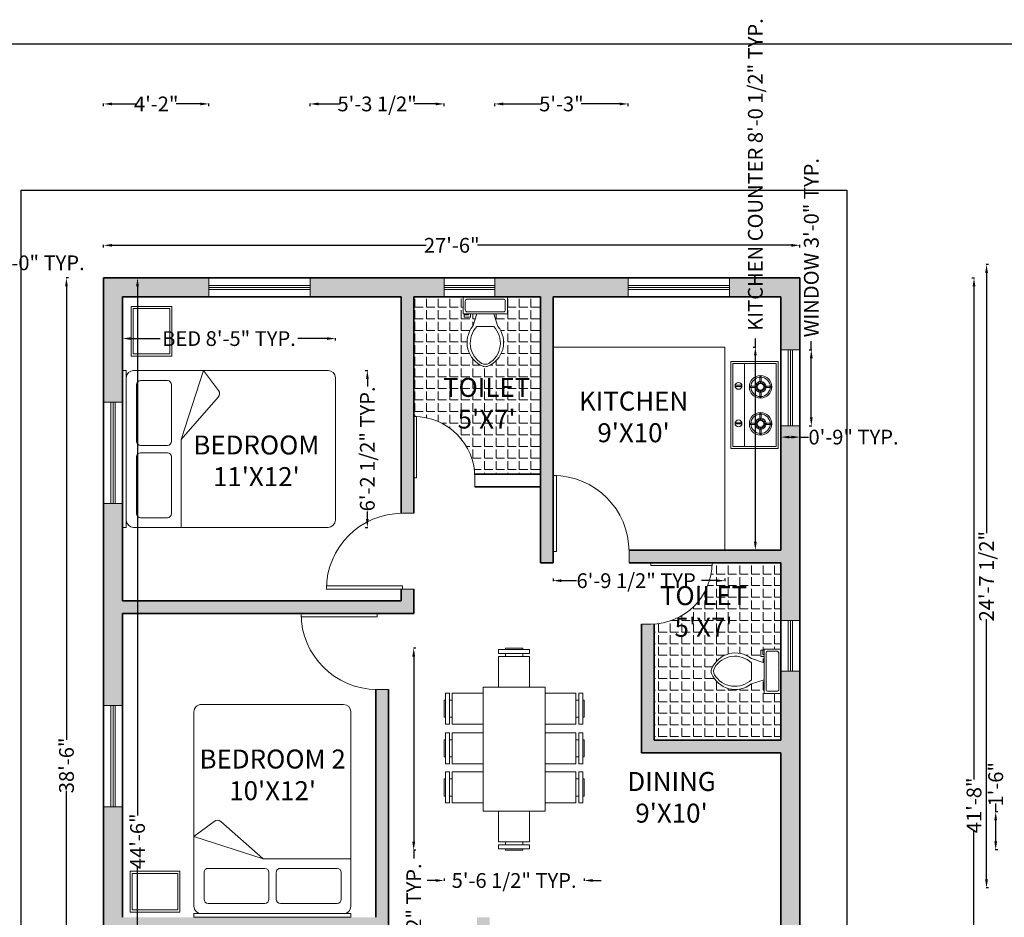
# Model space of a CAD drawing. Units: inches. Extents: x -80 to 1461, y -1239 to 153.
# Tile 5 of 6: x 358 to 824, y -273 to 153. Entities that reach past the tile are written whole.
import ezdxf

# ---------------------------------------------------------------- set-up
doc = ezdxf.new("R2010")
doc.units = ezdxf.units.IN
doc.header["$MEASUREMENT"] = 0
for name, color, linetype, lineweight in [('A-ANNO-DIMS', 2, 'Continuous', 18), ('A-ANNO-TTLB', 7, 'Continuous', 25), ('A-AREA-IDEN', 7, 'Continuous', 18), ('A-EQPM', 8, 'Continuous', 18), ('A-FLOR-FIXT', 9, 'Continuous', 18), ('A-FLOR-PATT', 143, 'Continuous', 13), ('A-FURN', 8, 'Continuous', 18), ('A-GLAZ', 4, 'Continuous', 18), ('A-WALL', 7, 'Continuous', 35), ('A-WALL-PATT', 8, 'Continuous', 13), ('DOOR', 32, 'Continuous', 18)]:
    doc.layers.add(name, color=color, linetype=linetype, lineweight=lineweight)
doc.styles.get("Standard").update_dxf_attribs({"font": 'arial.ttf'})
doc.dimstyles.get("Standard").update_dxf_attribs({"dimtxt": 7, "dimasz": 4, "dimexe": 0.18, "dimexo": 0.0625, "dimgap": 0.09, "dimtad": 0, "dimdec": 0, "dimzin": 0, "dimdsep": 46, "dimlunit": 3, "dimtxsty": 'Standard', "dimcen": 0.09, "dimadec": 0, "dimazin": 0, "dimtfac": 1, "dimtdec": 0, "dimtofl": 0, "dimtmove": 0, "dimatfit": 3, "dimfxl": 1, "dimfxlon": 1, "dimtolj": 1, "dimtzin": 0, "dimarcsym": 0})

# ---------------------------------------------------------------- blocks, each defined once
blk = doc.blocks.new('*U2')
for p, q in [((0, 0), (0, -6)), ((40, 0), (40, -6))]:
    blk.add_line(p, q)
blk.add_lwpolyline([(0, 0), (0, 40), (1.75, 40), (1.75, 0)], close=True)
blk.add_arc((0, 0), 40, 0, 90)
blk = doc.blocks.new('A$C164346CA')
for p, q in [((0, 2.035), (0, 2)), ((1.5, 2.035), (0, 2.035)), ((1.5, 2), (0, 2)), ((1.5, 2), (1.5, 2.035)), ((0, 1.93), (0, 0.07)), ((0.6731, 1.9024), (0.1319, 1.9024)), ((1.364, 1.9024), (0.8228, 1.9024)), ((1.5, 0.07), (1.5, 1.93)), ((0.0919, 1.8624), (0.0919, 1.6069)), ((0.7131, 1.6069), (0.7131, 1.8624)), ((0.7828, 1.8624), (0.7828, 1.6069)), ((1.404, 1.6069), (1.404, 1.8624)), ((0.1319, 1.5669), (0.6731, 1.5669)), ((0.8228, 1.5669), (1.364, 1.5669)), ((0.8395, 1.4761), (0, 1.4761)), ((0.8395, 1.4761), (1.2448, 1.12)), ((1.5, 1.2611), (0.8395, 1.4761)), ((1.3077, 1.1175), (1.5, 1.2611)), ((0.07, 0), (1.43, 0))]:
    blk.add_line(p, q)
for centre, radius, start, end in [((0.07, 1.93), 0.07, 90, 180), ((1.43, 1.93), 0.07, 0, 90), ((0.1319, 1.8624), 0.04, 90, 180), ((0.6731, 1.8624), 0.04, 0, 90), ((0.8228, 1.8624), 0.04, 90, 180), ((1.364, 1.8624), 0.04, 0, 90), ((0.1319, 1.6069), 0.04, 180, 270), ((0.6731, 1.6069), 0.04, 270, 0), ((0.8228, 1.6069), 0.04, 180, 270), ((1.364, 1.6069), 0.04, 270, 0), ((1.2778, 1.1575), 0.05, 228.69584, 306.75789), ((0.07, 0.07), 0.07, 180, 270), ((1.43, 0.07), 0.07, 270, 0)]:
    blk.add_arc(centre, radius, start, end)
blk = doc.blocks.new('*U5')
for p, q in [((241, -152), (241, -51)), ((-254, -216), (-203, -216)), ((-254, -241), (-254, -216)), ((-203, -216), (-203, -203)), ((-178, -203), (-178, -241)), ((-102, -203), (-152, -356)), ((102, -203), (152, -356)), ((-178, -241), (-254, -241)), ((102, -356), (-102, -356))]:
    blk.add_line(p, q)
blk.add_lwpolyline([(267, -203), (267, 0), (-267, 0), (-267, -203)], close=True)
for points in [[(-241, -51), (-241, -152)], [(216, -25), (-216, -25)], [(-216, -178), (216, -178)]]:
    blk.add_lwpolyline(points)
for centre, radius, start, end in [((-219, -48), 22.5, 81.8699, 188.1301), ((219, -48), 22.5, 351.8699, 98.1301), ((-219, -156), 22.5, 171.8699, 278.1301), ((219, -156), 22.5, 261.8699, 8.1301), ((89, -548), 309, 141.4691, 247.9714), ((107, -554), 288, 136.3677, 238.9468), ((-89, -548), 309, 292.0284, 38.5307), ((-107, -554), 288, 301.053, 43.6321), ((0, -708), 102, 245.7318, 294.2682), ((0, -737), 102, 254.8605, 285.1395)]:
    blk.add_arc(centre, radius, start, end)
blk = doc.blocks.new('A$C06E242FC')
for p, q in [((0, 455.6), (0.5, 456.1)), ((0, 455.6), (0, 0.5)), ((838.9, 456.1), (0.5, 456.1)), ((20, 435.6), (20.5, 436.1)), ((20, 435.6), (20, 20.5)), ((818.9, 436.1), (20.5, 436.1)), ((237.3, 411.5), (237.3, 356.2)), ((248.9, 411.5), (237.3, 411.5)), ((248.9, 356.2), (248.9, 411.5)), ((599.3, 411.5), (610.9, 411.5)), ((599.3, 411.5), (599.3, 356.2)), ((610.9, 356.2), (610.9, 411.5)), ((819.4, 435.6), (818.9, 436.1)), ((819.4, 20.5), (819.4, 435.6)), ((838.9, 456.1), (839.4, 455.6)), ((839.4, 0.5), (839.4, 455.6)), ((20, 324.4), (819.4, 324.4)), ((237.3, 356.2), (248.9, 356.2)), ((599.3, 356.2), (610.9, 356.2)), ((232.7, 272.7), (232.7, 214)), ((244.9, 272.7), (232.7, 272.7)), ((232.7, 214), (244.9, 214)), ((244.9, 214), (244.9, 272.7)), ((588.1, 272.7), (588.1, 214)), ((600.3, 272.7), (588.1, 272.7)), ((588.1, 214), (600.3, 214)), ((600.3, 214), (600.3, 272.7)), ((136.3, 176), (136.3, 163.8)), ((194.9, 176), (136.3, 176)), ((136.3, 163.8), (194.9, 163.8)), ((194.9, 163.8), (194.9, 176)), ((245.2, 126.1), (233, 126.1)), ((233, 126.1), (233, 67.4)), ((245.2, 67.4), (245.2, 126.1)), ((282.9, 176.3), (282.9, 164.1)), ((341.6, 176.3), (282.9, 176.3)), ((282.9, 164.1), (341.6, 164.1)), ((341.6, 164.1), (341.6, 176.3)), ((550.3, 176), (491.7, 176)), ((491.7, 176), (491.7, 163.8)), ((491.7, 163.8), (550.3, 163.8)), ((550.3, 163.8), (550.3, 176)), ((600.6, 126.1), (588.3, 126.1)), ((588.3, 126.1), (588.3, 67.4)), ((600.6, 67.4), (600.6, 126.1)), ((638.3, 176.3), (638.3, 164.1)), ((697, 176.3), (638.3, 176.3)), ((638.3, 164.1), (697, 164.1)), ((697, 164.1), (697, 176.3)), ((0, 0.5), (0.5, 0)), ((20, 20.5), (20.5, 20)), ((20.5, 20), (818.9, 20)), ((233, 67.4), (245.2, 67.4)), ((588.3, 67.4), (600.6, 67.4)), ((818.9, 20), (819.4, 20.5)), ((838.9, 0), (839.4, 0.5)), ((0.5, 0), (838.9, 0))]:
    blk.add_line(p, q)
for centre, radius in [((242, 382.9), 33.3), ((604.1, 382.9), 33.3), ((238.9, 170.1), 108.3), ((238.9, 170.1), 93.3), ((238.9, 170.1), 52.6), ((205.3, 189.5), 4.84), ((238.9, 170.1), 32.6), ((219.5, 203.7), 4.84), ((238.9, 208.9), 4.84), ((258.4, 203.7), 4.84), ((272.6, 189.5), 4.84), ((594.3, 170.1), 108.3), ((594.3, 170.1), 93.3), ((594.3, 170.1), 52.6), ((560.7, 189.5), 4.84), ((594.3, 170.1), 32.6), ((574.9, 203.7), 4.84), ((594.3, 208.9), 4.84), ((613.7, 203.7), 4.84), ((628, 189.5), 4.84), ((200.1, 170.1), 4.84), ((205.3, 150.6), 4.84), ((219.5, 136.4), 4.84), ((238.9, 131.2), 4.84), ((258.4, 136.4), 4.84), ((272.6, 150.6), 4.84), ((277.8, 170.1), 4.84), ((555.5, 170.1), 4.84), ((560.7, 150.6), 4.84), ((574.9, 136.4), 4.84), ((594.3, 131.2), 4.84), ((613.7, 136.4), 4.84), ((628, 150.6), 4.84), ((633.2, 170.1), 4.84)]:
    blk.add_circle(centre, radius)
blk = doc.blocks.new('A$C4C0603CD')
for p, q in [((1.106, 2.02), (0.656, 2.02)), ((0.656, 2.02), (0.656, 1.96)), ((1.006, 2.04), (0.756, 2.04)), ((0.756, 2.04), (0.756, 2.02)), ((1.006, 2.02), (1.006, 2.04)), ((1.106, 1.96), (1.106, 2.02)), ((1.232, 2.02), (1.232, 1.96)), ((1.684, 2.02), (1.232, 2.02)), ((1.584, 2.04), (1.334, 2.04)), ((1.334, 2.04), (1.334, 2.02)), ((1.584, 2.02), (1.584, 2.04)), ((1.684, 1.96), (1.684, 2.02)), ((1.802, 2.02), (1.802, 1.96)), ((2.252, 2.02), (1.802, 2.02)), ((2.152, 2.04), (1.902, 2.04)), ((1.902, 2.04), (1.902, 2.02)), ((2.152, 2.02), (2.152, 2.04)), ((2.252, 1.96), (2.252, 2.02)), ((1.106, 1.96), (0.656, 1.96)), ((0.656, 1.92), (0.656, 1.47)), ((1.106, 1.92), (0.656, 1.92)), ((0.756, 1.96), (0.756, 1.92)), ((1.006, 1.92), (1.006, 1.96)), ((1.106, 1.47), (1.106, 1.92)), ((1.684, 1.96), (1.232, 1.96)), ((1.232, 1.92), (1.232, 1.47)), ((1.684, 1.92), (1.232, 1.92)), ((1.334, 1.96), (1.334, 1.92)), ((1.584, 1.92), (1.584, 1.96)), ((1.684, 1.47), (1.684, 1.92)), ((2.252, 1.96), (1.802, 1.96)), ((1.802, 1.92), (1.802, 1.47)), ((2.252, 1.92), (1.802, 1.92)), ((1.902, 1.96), (1.902, 1.92)), ((2.152, 1.92), (2.152, 1.96)), ((2.252, 1.47), (2.252, 1.92)), ((0.57, 1.47), (0.57, 0.57)), ((2.37, 1.47), (0.57, 1.47)), ((0.656, 1.47), (1.106, 1.47)), ((1.107, 1.47), (1.684, 1.47)), ((1.802, 1.47), (2.252, 1.47)), ((2.37, 1.47), (2.37, 0.57)), ((0.02, 1.245), (0.02, 0.795)), ((0.08, 1.245), (0.02, 1.245)), ((0.08, 1.245), (0.08, 0.795)), ((0.12, 1.245), (0.12, 0.795)), ((0.57, 1.245), (0.12, 1.245)), ((0.57, 0.795), (0.57, 1.245)), ((2.37, 1.245), (2.37, 0.795)), ((2.82, 1.245), (2.37, 1.245)), ((2.82, 0.795), (2.82, 1.245)), ((2.86, 0.795), (2.86, 1.245)), ((2.92, 1.245), (2.86, 1.245)), ((2.92, 0.795), (2.92, 1.245)), ((0, 1.145), (0, 0.895)), ((0.02, 1.145), (0, 1.145)), ((0.12, 1.145), (0.08, 1.145)), ((2.86, 1.145), (2.82, 1.145)), ((2.94, 1.145), (2.92, 1.145)), ((2.94, 0.895), (2.94, 1.145)), ((0, 0.895), (0.02, 0.895)), ((0.08, 0.895), (0.12, 0.895)), ((2.82, 0.895), (2.86, 0.895)), ((2.92, 0.895), (2.94, 0.895)), ((0.02, 0.795), (0.08, 0.795)), ((0.12, 0.795), (0.57, 0.795)), ((2.37, 0.795), (2.82, 0.795)), ((2.86, 0.795), (2.92, 0.795)), ((0.57, 0.57), (2.37, 0.57)), ((1.106, 0.57), (0.656, 0.57)), ((0.656, 0.57), (0.656, 0.12)), ((1.106, 0.12), (1.106, 0.57)), ((1.684, 0.57), (1.232, 0.57)), ((1.232, 0.57), (1.232, 0.12)), ((1.684, 0.12), (1.684, 0.57)), ((2.252, 0.57), (1.802, 0.57)), ((1.802, 0.57), (1.802, 0.12)), ((2.252, 0.12), (2.252, 0.57)), ((0.656, 0.12), (1.106, 0.12)), ((0.656, 0.08), (1.106, 0.08)), ((0.656, 0.08), (0.656, 0.02)), ((0.656, 0.02), (1.106, 0.02)), ((0.756, 0.12), (0.756, 0.08)), ((0.756, 0.02), (0.756, 0)), ((0.756, 0), (1.006, 0)), ((1.006, 0.08), (1.006, 0.12)), ((1.006, 0), (1.006, 0.02)), ((1.106, 0.02), (1.106, 0.08)), ((1.232, 0.12), (1.684, 0.12)), ((1.232, 0.08), (1.684, 0.08)), ((1.232, 0.08), (1.232, 0.02)), ((1.232, 0.02), (1.684, 0.02)), ((1.334, 0.12), (1.334, 0.08)), ((1.334, 0.02), (1.334, 0)), ((1.334, 0), (1.584, 0)), ((1.584, 0.08), (1.584, 0.12)), ((1.584, 0), (1.584, 0.02)), ((1.684, 0.02), (1.684, 0.08)), ((1.802, 0.12), (2.252, 0.12)), ((1.802, 0.08), (2.252, 0.08)), ((1.802, 0.08), (1.802, 0.02)), ((1.802, 0.02), (2.252, 0.02)), ((1.902, 0.12), (1.902, 0.08)), ((1.902, 0.02), (1.902, 0)), ((1.902, 0), (2.152, 0)), ((2.152, 0.08), (2.152, 0.12)), ((2.152, 0), (2.152, 0.02)), ((2.252, 0.02), (2.252, 0.08))]:
    blk.add_line(p, q)
blk = doc.blocks.new('*D13')
at = {"layer": 'A-ANNO-DIMS', "color": 0, "lineweight": -2, "transparency": 16777216}
for p, q in [((397.42, 44.81), (397.42, 45.99)), ((401.42, 45.81), (550.24, 45.81)), ((723.42, 45.81), (574.59, 45.81)), ((727.42, 44.81), (727.42, 45.99))]:
    blk.add_line(p, q, dxfattribs=at)
at = {"layer": 'A-ANNO-DIMS', "color": 0, "transparency": 16777216}
for points in [[(401.42, 46.47), (401.42, 45.14), (397.42, 45.81)], [(723.42, 46.47), (723.42, 45.14), (727.42, 45.81)]]:
    blk.add_solid(points, dxfattribs=at)
at = {"layer": 'Defpoints', "color": 0, "transparency": 16777216}
for p in [(727.42, 45.81), (397.42, 30.32), (727.42, 30.32)]:
    blk.add_point(p, dxfattribs=at)
at = {"layer": 'A-ANNO-DIMS', "color": 0, "transparency": 16777216, "insert": (562.42, 45.81), "char_height": 7, "attachment_point": 5}
blk.add_mtext('\\A1;27\'-6"', dxfattribs=at)
blk = doc.blocks.new('*D14')
at = {"layer": 'A-ANNO-DIMS', "color": 0, "lineweight": -2, "transparency": 16777216}
for p, q in [((380.82, 30.32), (379.64, 30.32)), ((379.82, 26.32), (379.82, -188.57)), ((379.82, -427.68), (379.82, -212.8)), ((380.82, -431.68), (379.64, -431.68))]:
    blk.add_line(p, q, dxfattribs=at)
at = {"layer": 'A-ANNO-DIMS', "color": 0, "transparency": 16777216}
for points in [[(379.15, 26.32), (380.48, 26.32), (379.82, 30.32)], [(379.15, -427.68), (380.48, -427.68), (379.82, -431.68)]]:
    blk.add_solid(points, dxfattribs=at)
at = {"layer": 'Defpoints', "color": 0, "transparency": 16777216}
for p in [(397.42, 30.32), (379.82, -431.68), (397.42, -431.68)]:
    blk.add_point(p, dxfattribs=at)
at = {"layer": 'A-ANNO-DIMS', "color": 0, "transparency": 16777216, "insert": (379.82, -200.68), "char_height": 7, "attachment_point": 5, "rotation": 90}
blk.add_mtext('\\A1;38\'-6"', dxfattribs=at)
blk = doc.blocks.new('*D21')
at = {"layer": 'A-ANNO-DIMS', "color": 0, "lineweight": -2, "transparency": 16777216}
for p, q in [((820.21, -222.68), (820.21, -218.68)), ((821.21, -222.68), (820.03, -222.68)), ((820.21, -236.68), (820.21, -226.68)), ((821.21, -240.68), (820.03, -240.68))]:
    blk.add_line(p, q, dxfattribs=at)
at = {"layer": 'A-ANNO-DIMS', "color": 0, "transparency": 16777216}
for points in [[(819.55, -226.68), (820.88, -226.68), (820.21, -222.68)], [(819.55, -236.68), (820.88, -236.68), (820.21, -240.68)]]:
    blk.add_solid(points, dxfattribs=at)
at = {"layer": 'Defpoints', "color": 0, "transparency": 16777216}
for p in [(820.21, -222.68), (841.26, -222.68), (838.26, -240.68)]:
    blk.add_point(p, dxfattribs=at)
at = {"layer": 'A-ANNO-DIMS', "color": 0, "transparency": 16777216, "insert": (820.21, -209.62), "char_height": 7, "attachment_point": 5, "rotation": 90}
blk.add_mtext('\\A1;1\'-6"', dxfattribs=at)
blk = doc.blocks.new('WIN-48IN')
for p, q in [((0, 9), (0, 0)), ((48, 9), (0, 9)), ((0, 5.5), (48, 5.5)), ((48, 0), (48, 9)), ((0, 4.5), (48, 4.5)), ((0, 3.5), (48, 3.5)), ((0, 0), (36, 0)), ((36, 0), (48, 0))]:
    blk.add_line(p, q)
blk = doc.blocks.new('WIN-24IN')
for p, q in [((0, 9), (0, 0)), ((0, 9), (24, 9)), ((0, 5.5), (24, 5.5)), ((24, 9), (24, 0)), ((0, 4.5), (24, 4.5)), ((0, 3.5), (24, 3.5)), ((0, 0), (24, 0))]:
    blk.add_line(p, q)
blk = doc.blocks.new('WIN-36IN')
for p, q in [((0, 36), (9, 36)), ((0, 36), (0, 0)), ((3.5, 0), (3.5, 36)), ((4.5, 0), (4.5, 36)), ((5.5, 0), (5.5, 36)), ((9, 0), (9, 36)), ((0, 0), (9, 0))]:
    blk.add_line(p, q)
blk = doc.blocks.new('NIGHTSTAND')
for points in [[(0, 19.36), (23.56, 19.36), (23.56, 0), (0, 0)], [(1, 18.36), (22.56, 18.36), (22.56, 1), (1, 1)]]:
    blk.add_lwpolyline(points, close=True)
blk = doc.blocks.new('COUNTER-L-PLAN')
for p, q in [((0, 96.29), (81.45, 96.29)), ((81.45, 96.29), (81.45, 0))]:
    blk.add_line(p, q)
blk = doc.blocks.new('*D36')
at = {"layer": 'A-ANNO-DIMS', "color": 0, "lineweight": -2, "transparency": 16777216}
for p, q in [((249.57, 36.52), (249.57, 37.7)), ((253.57, 37.52), (293.57, 37.52)), ((297.57, 36.52), (297.57, 37.7)), ((297.57, 37.52), (301.57, 37.52))]:
    blk.add_line(p, q, dxfattribs=at)
at = {"layer": 'A-ANNO-DIMS', "color": 0, "transparency": 16777216}
for points in [[(253.57, 38.18), (253.57, 36.85), (249.57, 37.52)], [(293.57, 38.18), (293.57, 36.85), (297.57, 37.52)]]:
    blk.add_solid(points, dxfattribs=at)
at = {"layer": 'Defpoints', "color": 0, "transparency": 16777216}
for p in [(297.57, 37.52), (249.57, 30.32), (297.57, 30.32)]:
    blk.add_point(p, dxfattribs=at)
at = {"layer": 'A-ANNO-DIMS', "color": 0, "transparency": 16777216, "insert": (345.95, 37.52), "char_height": 7, "attachment_point": 5}
blk.add_mtext('\\A1;WINDOW 4\'-0" TYP.', dxfattribs=at)
blk = doc.blocks.new('*D40')
at = {"layer": 'A-ANNO-DIMS', "color": 0, "lineweight": -2, "transparency": 16777216}
for p, q in [((732.82, -3.69), (732.82, 0.31)), ((731.82, -3.69), (733, -3.69)), ((732.82, -35.69), (732.82, -7.69)), ((731.82, -39.69), (733, -39.69))]:
    blk.add_line(p, q, dxfattribs=at)
at = {"layer": 'A-ANNO-DIMS', "color": 0, "transparency": 16777216}
for points in [[(732.15, -7.69), (733.48, -7.69), (732.82, -3.69)], [(732.15, -35.69), (733.48, -35.69), (732.82, -39.69)]]:
    blk.add_solid(points, dxfattribs=at)
at = {"layer": 'Defpoints', "color": 0, "transparency": 16777216}
for p in [(727.42, -3.69), (732.82, -3.69), (727.42, -39.69)]:
    blk.add_point(p, dxfattribs=at)
at = {"layer": 'A-ANNO-DIMS', "color": 0, "transparency": 16777216, "insert": (732.82, 44.69), "char_height": 7, "attachment_point": 5, "rotation": 90}
blk.add_mtext('\\A1;WINDOW 3\'-0" TYP.', dxfattribs=at)
blk = doc.blocks.new('*D41')
at = {"layer": 'A-ANNO-DIMS', "color": 0, "lineweight": -2, "transparency": 16777216}
for p, q in [((718.42, -44.09), (718.42, -45.27)), ((722.42, -45.09), (723.42, -45.09)), ((727.42, -44.09), (727.42, -45.27)), ((727.42, -45.09), (731.42, -45.09))]:
    blk.add_line(p, q, dxfattribs=at)
at = {"layer": 'A-ANNO-DIMS', "color": 0, "transparency": 16777216}
for points in [[(722.42, -44.42), (722.42, -45.76), (718.42, -45.09)], [(723.42, -44.42), (723.42, -45.76), (727.42, -45.09)]]:
    blk.add_solid(points, dxfattribs=at)
at = {"layer": 'Defpoints', "color": 0, "transparency": 16777216}
for p in [(718.42, -39.69), (727.42, -39.69), (727.42, -45.09)]:
    blk.add_point(p, dxfattribs=at)
at = {"layer": 'A-ANNO-DIMS', "color": 0, "transparency": 16777216, "insert": (752.84, -45.09), "char_height": 7, "attachment_point": 5}
blk.add_mtext('\\A1;0\'-9" TYP.', dxfattribs=at)
blk = doc.blocks.new('*D46')
at = {"layer": 'A-ANNO-DIMS', "color": 0, "lineweight": -2, "transparency": 16777216}
for p, q in [((406.42, 0.62), (406.42, 1.8)), ((410.42, 1.62), (424.17, 1.62)), ((503.29, 1.62), (489.53, 1.62)), ((507.29, 0.62), (507.29, 1.8))]:
    blk.add_line(p, q, dxfattribs=at)
at = {"layer": 'A-ANNO-DIMS', "color": 0, "transparency": 16777216}
for points in [[(410.42, 2.29), (410.42, 0.96), (406.42, 1.62)], [(503.29, 2.29), (503.29, 0.96), (507.29, 1.62)]]:
    blk.add_solid(points, dxfattribs=at)
at = {"layer": 'Defpoints', "color": 0, "transparency": 16777216}
for p in [(406.42, 1.62), (406.42, -13.51), (507.29, -13.51)]:
    blk.add_point(p, dxfattribs=at)
at = {"layer": 'A-ANNO-DIMS', "color": 0, "transparency": 16777216, "insert": (456.85, 1.62), "char_height": 7, "attachment_point": 5}
blk.add_mtext('\\A1;BED 8\'-5" TYP.', dxfattribs=at)
blk = doc.blocks.new('*D47')
at = {"layer": 'A-ANNO-DIMS', "color": 0, "lineweight": -2, "transparency": 16777216}
for p, q in [((521.42, -13.51), (522.6, -13.51)), ((522.42, -17.51), (522.42, -21.09)), ((522.42, -83.86), (522.42, -80.28)), ((521.42, -87.86), (522.6, -87.86))]:
    blk.add_line(p, q, dxfattribs=at)
at = {"layer": 'A-ANNO-DIMS', "color": 0, "transparency": 16777216}
for points in [[(521.75, -17.51), (523.08, -17.51), (522.42, -13.51)], [(521.75, -83.86), (523.08, -83.86), (522.42, -87.86)]]:
    blk.add_solid(points, dxfattribs=at)
at = {"layer": 'Defpoints', "color": 0, "transparency": 16777216}
for p in [(507.29, -13.51), (522.42, -13.51), (507.29, -87.86)]:
    blk.add_point(p, dxfattribs=at)
at = {"layer": 'A-ANNO-DIMS', "color": 0, "transparency": 16777216, "insert": (522.42, -50.68), "char_height": 7, "attachment_point": 5, "rotation": 90}
blk.add_mtext('\\A1;6\'-2 1/2" TYP.', dxfattribs=at)
blk = doc.blocks.new('*D52')
at = {"layer": 'A-ANNO-DIMS', "color": 0, "lineweight": -2, "transparency": 16777216}
for p, q in [((545.39, -145.12), (544.21, -145.12)), ((544.39, -149.12), (544.39, -236.86)), ((545.39, -240.86), (544.21, -240.86)), ((544.39, -240.86), (544.39, -244.86))]:
    blk.add_line(p, q, dxfattribs=at)
at = {"layer": 'A-ANNO-DIMS', "color": 0, "transparency": 16777216}
for points in [[(543.72, -149.12), (545.06, -149.12), (544.39, -145.12)], [(543.72, -236.86), (545.06, -236.86), (544.39, -240.86)]]:
    blk.add_solid(points, dxfattribs=at)
at = {"layer": 'Defpoints', "color": 0, "transparency": 16777216}
for p in [(558.75, -145.12), (544.39, -240.86), (558.75, -240.86)]:
    blk.add_point(p, dxfattribs=at)
at = {"layer": 'A-ANNO-DIMS', "color": 0, "transparency": 16777216, "insert": (544.39, -306.33), "char_height": 7, "attachment_point": 5, "rotation": 90}
blk.add_mtext('\\A1;DINING SET 7\'-11 1/2" TYP.', dxfattribs=at)
blk = doc.blocks.new('*D53')
at = {"layer": 'A-ANNO-DIMS', "color": 0, "lineweight": -2, "transparency": 16777216}
for p, q in [((554.75, -255.23), (550.75, -255.23)), ((558.75, -254.23), (558.75, -255.41)), ((625.19, -254.23), (625.19, -255.41)), ((629.19, -255.23), (633.19, -255.23))]:
    blk.add_line(p, q, dxfattribs=at)
at = {"layer": 'A-ANNO-DIMS', "color": 0, "transparency": 16777216}
for points in [[(554.75, -254.56), (554.75, -255.89), (558.75, -255.23)], [(629.19, -254.56), (629.19, -255.89), (625.19, -255.23)]]:
    blk.add_solid(points, dxfattribs=at)
at = {"layer": 'Defpoints', "color": 0, "transparency": 16777216}
for p in [(558.75, -240.86), (625.19, -240.86), (625.19, -255.23)]:
    blk.add_point(p, dxfattribs=at)
at = {"layer": 'A-ANNO-DIMS', "color": 0, "transparency": 16777216, "insert": (591.97, -255.23), "char_height": 7, "attachment_point": 5}
blk.add_mtext('\\A1;5\'-6 1/2" TYP.', dxfattribs=at)
blk = doc.blocks.new('*D60')
at = {"layer": 'A-ANNO-DIMS', "color": 0, "lineweight": -2, "transparency": 16777216}
for p, q in [((706.3, -2.4), (706.3, 1.6)), ((705.3, -2.4), (706.48, -2.4)), ((706.3, -94.68), (706.3, -6.4)), ((705.3, -98.68), (706.48, -98.68))]:
    blk.add_line(p, q, dxfattribs=at)
at = {"layer": 'A-ANNO-DIMS', "color": 0, "transparency": 16777216}
for points in [[(705.64, -6.4), (706.97, -6.4), (706.3, -2.4)], [(705.64, -94.68), (706.97, -94.68), (706.3, -98.68)]]:
    blk.add_solid(points, dxfattribs=at)
at = {"layer": 'Defpoints', "color": 0, "transparency": 16777216}
for p in [(691.86, -2.4), (706.3, -2.4), (691.86, -98.68)]:
    blk.add_point(p, dxfattribs=at)
at = {"layer": 'A-ANNO-DIMS', "color": 0, "transparency": 16777216, "insert": (706.3, 79.38), "char_height": 7, "attachment_point": 5, "rotation": 90}
blk.add_mtext('\\A1;KITCHEN COUNTER 8\'-0 1/2" TYP.', dxfattribs=at)
blk = doc.blocks.new('*D61')
at = {"layer": 'A-ANNO-DIMS', "color": 0, "lineweight": -2, "transparency": 16777216}
for p, q in [((610.42, -112.13), (610.42, -113.31)), ((614.42, -113.13), (621.54, -113.13)), ((687.86, -113.13), (680.74, -113.13)), ((691.86, -112.13), (691.86, -113.31))]:
    blk.add_line(p, q, dxfattribs=at)
at = {"layer": 'A-ANNO-DIMS', "color": 0, "transparency": 16777216}
for points in [[(614.42, -112.46), (614.42, -113.79), (610.42, -113.13)], [(687.86, -112.46), (687.86, -113.79), (691.86, -113.13)]]:
    blk.add_solid(points, dxfattribs=at)
at = {"layer": 'Defpoints', "color": 0, "transparency": 16777216}
for p in [(610.42, -98.68), (691.86, -98.68), (691.86, -113.13)]:
    blk.add_point(p, dxfattribs=at)
at = {"layer": 'A-ANNO-DIMS', "color": 0, "transparency": 16777216, "insert": (651.14, -113.13), "char_height": 7, "attachment_point": 5}
blk.add_mtext('\\A1;6\'-9 1/2" TYP.', dxfattribs=at)
blk = doc.blocks.new('*D63')
at = {"layer": 'A-ANNO-DIMS', "color": 0, "lineweight": -2, "transparency": 16777216}
for p, q in [((816.86, 36.65), (815.68, 36.65)), ((815.86, 32.65), (815.86, -90.69)), ((815.86, -254.68), (815.86, -131.34)), ((816.86, -258.68), (815.68, -258.68))]:
    blk.add_line(p, q, dxfattribs=at)
at = {"layer": 'A-ANNO-DIMS', "color": 0, "transparency": 16777216}
for points in [[(815.2, 32.65), (816.53, 32.65), (815.86, 36.65)], [(815.2, -254.68), (816.53, -254.68), (815.86, -258.68)]]:
    blk.add_solid(points, dxfattribs=at)
at = {"layer": 'Defpoints', "color": 0, "transparency": 16777216}
for p in [(815.86, 36.65), (847.26, 36.65), (835.26, -258.68)]:
    blk.add_point(p, dxfattribs=at)
at = {"layer": 'A-ANNO-DIMS', "color": 0, "transparency": 16777216, "insert": (815.86, -111.02), "char_height": 7, "attachment_point": 5, "rotation": 90}
blk.add_mtext('\\A1;24\'-7 1/2"', dxfattribs=at)
blk = doc.blocks.new('*D72')
at = {"layer": 'A-ANNO-DIMS', "color": 0, "lineweight": -2, "transparency": 16777216}
for p, q in [((412.49, 30.32), (413.67, 30.32)), ((413.49, 26.32), (413.49, -224.38)), ((413.49, -499.58), (413.49, -248.89)), ((412.49, -503.58), (413.67, -503.58))]:
    blk.add_line(p, q, dxfattribs=at)
at = {"layer": 'A-ANNO-DIMS', "color": 0, "transparency": 16777216}
for points in [[(412.82, 26.32), (414.16, 26.32), (413.49, 30.32)], [(412.82, -499.58), (414.16, -499.58), (413.49, -503.58)]]:
    blk.add_solid(points, dxfattribs=at)
at = {"layer": 'Defpoints', "color": 0, "transparency": 16777216}
for p in [(330.99, 30.32), (183.99, -503.58), (413.49, -503.58)]:
    blk.add_point(p, dxfattribs=at)
at = {"layer": 'A-ANNO-DIMS', "color": 0, "transparency": 16777216, "insert": (413.49, -236.63), "char_height": 7, "attachment_point": 5, "rotation": 90}
blk.add_mtext('\\A1;44\'-6"', dxfattribs=at)
blk = doc.blocks.new('*D73')
at = {"layer": 'A-ANNO-DIMS', "color": 0, "lineweight": -2, "transparency": 16777216}
for p, q in [((808.92, 30.32), (810.1, 30.32)), ((809.92, 26.32), (809.92, -207.38)), ((809.92, -465.58), (809.92, -231.89)), ((808.92, -469.58), (810.1, -469.58))]:
    blk.add_line(p, q, dxfattribs=at)
at = {"layer": 'A-ANNO-DIMS', "color": 0, "transparency": 16777216}
for points in [[(809.25, 26.32), (810.58, 26.32), (809.92, 30.32)], [(809.25, -465.58), (810.58, -465.58), (809.92, -469.58)]]:
    blk.add_solid(points, dxfattribs=at)
at = {"layer": 'Defpoints', "color": 0, "transparency": 16777216}
for p in [(727.42, 30.32), (809.92, 30.32), (580.42, -469.58)]:
    blk.add_point(p, dxfattribs=at)
at = {"layer": 'A-ANNO-DIMS', "color": 0, "transparency": 16777216, "insert": (809.92, -219.63), "char_height": 7, "attachment_point": 5, "rotation": 90}
blk.add_mtext('\\A1;41\'-8"', dxfattribs=at)
blk = doc.blocks.new('*D77')
at = {"layer": 'A-ANNO-DIMS', "color": 0, "lineweight": -2, "transparency": 16777216}
for p, q in [((610.42, -500.08), (610.42, -501.26)), ((614.42, -501.08), (619.02, -501.08)), ((642.42, -501.08), (637.81, -501.08)), ((646.42, -500.08), (646.42, -501.26))]:
    blk.add_line(p, q, dxfattribs=at)
at = {"layer": 'A-ANNO-DIMS', "color": 0, "transparency": 16777216}
for points in [[(614.42, -500.42), (614.42, -501.75), (610.42, -501.08)], [(642.42, -500.42), (642.42, -501.75), (646.42, -501.08)]]:
    blk.add_solid(points, dxfattribs=at)
at = {"layer": 'Defpoints', "color": 0, "transparency": 16777216}
for p in [(610.42, -104.68), (646.42, -104.68), (646.42, -501.08)]:
    blk.add_point(p, dxfattribs=at)
at = {"layer": 'A-ANNO-DIMS', "color": 0, "transparency": 16777216, "insert": (628.42, -501.08), "char_height": 7, "attachment_point": 5}
blk.add_mtext('\\A1;3\'-0"', dxfattribs=at)
blk = doc.blocks.new('*D78')
at = {"layer": 'A-ANNO-DIMS', "color": 0, "lineweight": -2, "transparency": 16777216}
for p, q in [((397.42, 111.82), (397.42, 113)), ((401.42, 112.82), (412.81, 112.82)), ((443.28, 112.82), (431.88, 112.82)), ((447.28, 111.82), (447.28, 113))]:
    blk.add_line(p, q, dxfattribs=at)
at = {"layer": 'A-ANNO-DIMS', "color": 0, "transparency": 16777216}
for points in [[(401.42, 113.48), (401.42, 112.15), (397.42, 112.82)], [(443.28, 113.48), (443.28, 112.15), (447.28, 112.82)]]:
    blk.add_solid(points, dxfattribs=at)
at = {"layer": 'Defpoints', "color": 0, "transparency": 16777216}
for p in [(447.28, 112.82), (397.42, 30.32), (447.28, 30.32)]:
    blk.add_point(p, dxfattribs=at)
at = {"layer": 'A-ANNO-DIMS', "color": 0, "transparency": 16777216, "insert": (422.35, 112.82), "char_height": 7, "attachment_point": 5}
blk.add_mtext('\\A1;4\'-2"', dxfattribs=at)
blk = doc.blocks.new('*D79')
at = {"layer": 'A-ANNO-DIMS', "color": 0, "lineweight": -2, "transparency": 16777216}
for p, q in [((495.28, 111.82), (495.28, 113)), ((499.28, 112.82), (509.49, 112.82)), ((554.8, 112.82), (544.59, 112.82)), ((558.8, 111.82), (558.8, 113))]:
    blk.add_line(p, q, dxfattribs=at)
at = {"layer": 'A-ANNO-DIMS', "color": 0, "transparency": 16777216}
for points in [[(499.28, 113.48), (499.28, 112.15), (495.28, 112.82)], [(554.8, 113.48), (554.8, 112.15), (558.8, 112.82)]]:
    blk.add_solid(points, dxfattribs=at)
at = {"layer": 'Defpoints', "color": 0, "transparency": 16777216}
for p in [(558.8, 112.82), (495.28, 30.32), (558.8, 30.32)]:
    blk.add_point(p, dxfattribs=at)
at = {"layer": 'A-ANNO-DIMS', "color": 0, "transparency": 16777216, "insert": (527.04, 112.82), "char_height": 7, "attachment_point": 5}
blk.add_mtext('\\A1;5\'-3 1/2"', dxfattribs=at)
blk = doc.blocks.new('*D80')
at = {"layer": 'A-ANNO-DIMS', "color": 0, "lineweight": -2, "transparency": 16777216}
for p, q in [((582.8, 111.82), (582.8, 113)), ((586.8, 112.82), (605, 112.82)), ((641.99, 112.82), (623.79, 112.82)), ((645.99, 111.82), (645.99, 113))]:
    blk.add_line(p, q, dxfattribs=at)
at = {"layer": 'A-ANNO-DIMS', "color": 0, "transparency": 16777216}
for points in [[(586.8, 113.48), (586.8, 112.15), (582.8, 112.82)], [(641.99, 113.48), (641.99, 112.15), (645.99, 112.82)]]:
    blk.add_solid(points, dxfattribs=at)
at = {"layer": 'Defpoints', "color": 0, "transparency": 16777216}
for p in [(645.99, 112.82), (582.8, 30.32), (645.99, 30.32)]:
    blk.add_point(p, dxfattribs=at)
at = {"layer": 'A-ANNO-DIMS', "color": 0, "transparency": 16777216, "insert": (614.39, 112.82), "char_height": 7, "attachment_point": 5}
blk.add_mtext('\\A1;5\'-3"', dxfattribs=at)

msp = doc.modelspace()

# ---------------------------------------------------------------- hatches: boundary and pattern name
at = {"layer": 'A-FLOR-PATT'}
h = msp.add_hatch(dxfattribs=at)
h.set_pattern_fill('ANGLE', color=256, scale=20)
h.set_pattern_definition([(0, (396.4254, 0), (0, 5.5), [4, -1.5]), (90, (396.4254, 0), (-5.5, 3e-16), [4, -1.5])])
h.paths.add_polyline_path([(604.42, 21.32), (588.82, 21.32), (588.82, 13.32), (582.32, 13.32), (584.32, 7.32, -0.501323), (579.36, -11.55, -0.132891), (577.27, -11.55, -0.501317), (572.32, 7.32), (574.32, 13.32), (571.32, 13.32), (571.32, 11.82), (568.32, 11.82), (568.32, 12.82), (570.32, 12.82), (570.32, 13.32), (567.82, 13.32), (567.82, 21.32), (558.8, 21.32), (544.42, 21.32), (544.42, -35.33), (545.68, -35.33), (545.68, -35.36, -0.38502), (573.37, -62.68), (604.42, -62.68)])
h.paths.add_polyline_path([(718.42, -104.68), (685.77, -104.68), (685.77, -105.95), (685.74, -105.95, -0.38502), (658.42, -133.64), (658.42, -188.68), (718.42, -188.68), (718.42, -166.56), (710.42, -166.56), (710.42, -160.06), (704.42, -162.06, -0.501323), (685.55, -157.1, -0.132891), (685.55, -155.01, -0.501317), (704.42, -150.06), (710.42, -152.06), (710.42, -149.06), (708.92, -149.06), (708.92, -146.06), (710.42, -146.06), (710.42, -145.56), (718.42, -145.56)])
at = {"layer": 'A-WALL-PATT'}
h = msp.add_hatch(color=256, dxfattribs=at)
h.dxf.hatch_style = 1
h.paths.add_polyline_path([(406.42, -76.5), (397.42, -76.5), (397.42, -172.33), (406.42, -172.33), (406.42, -128.68), (544.42, -128.68), (544.42, -117.2), (539.02, -117.2), (538.42, -117.2), (538.42, -122.68), (406.42, -122.68)])
h.paths.add_polyline_path([(447.28, 30.32), (397.42, 30.32), (397.42, -28.5), (406.42, -28.5), (406.42, -13.51), (406.42, 21.32), (447.28, 21.32)])
h = msp.add_hatch(color=256, dxfattribs=at)
h.dxf.hatch_style = 1
h.paths.add_polyline_path([(558.8, 30.32), (495.28, 30.32), (495.28, 21.32), (538.42, 21.32), (538.42, -81.2, -0.004167), (539.02, -81.2), (544.42, -81.2), (544.42, 21.32), (558.8, 21.32)])
h.paths.add_polyline_path([(727.42, 30.32), (693.99, 30.32), (693.99, 21.32), (718.42, 21.32), (718.42, -3.69), (727.42, -3.69)])
h.paths.add_polyline_path([(645.99, 30.32), (582.8, 30.32), (582.8, 21.32), (588.82, 21.32), (604.42, 21.32), (604.42, -104.68), (610.42, -104.68), (610.42, -99.28), (610.42, -63.28), (610.42, 21.32), (645.99, 21.32)])
h.paths.add_polyline_path([(727.42, -39.69), (718.42, -39.69), (718.42, -98.68), (646.41, -98.68, -0.004167), (646.42, -99.28), (646.42, -104.68), (718.42, -104.68), (718.42, -132.06), (727.42, -132.06)])
h.paths.add_polyline_path([(727.42, -156.06), (718.42, -156.06), (718.42, -166.56), (718.42, -188.68), (658.42, -188.68), (658.42, -133.64, -0.014233), (656.77, -133.68), (652.42, -133.68), (652.42, -194.68), (718.42, -194.68), (718.42, -372.42), (702.59, -372.42), (702.59, -381.42), (727.42, -381.42)])
h = msp.add_hatch(color=256, dxfattribs=at)
h.dxf.hatch_style = 1
h.paths.add_polyline_path([(580.42, -272.68), (574.42, -272.68), (574.42, -422.68), (560.05, -422.68), (560.05, -426.28), (560.05, -431.68), (580.42, -431.68)])
h.paths.add_polyline_path([(406.42, -220.33), (397.42, -220.33), (397.42, -328.45), (406.42, -328.45), (406.42, -278.68), (532.42, -278.68), (532.42, -272.68), (406.42, -272.68)])
h.paths.add_polyline_path([(532.42, -164.68), (527.02, -164.68, -0.004167), (526.42, -164.68), (526.42, -272.68), (532.42, -272.68)])
h.paths.add_polyline_path([(524.05, -426.28, -0.025047), (524.23, -422.68), (469.7, -422.68), (469.7, -431.68), (524.05, -431.68)])
h.paths.add_polyline_path([(421.7, -422.68), (406.42, -422.68), (406.42, -376.45), (397.42, -376.45), (397.42, -431.68), (421.7, -431.68)])

# ---------------------------------------------------------------- linework, layer by layer
at = {"layer": 'A-ANNO-TTLB'}
for points in [[(-79.81, 141.36), (1461.09, 141.36), (1461.09, -1239.28), (-79.81, -1239.28)], [(358.28, 71.88), (749.61, 71.88), (749.61, -556.04), (358.28, -556.04)]]:
    msp.add_lwpolyline(points, close=True, dxfattribs=at)
at = {"layer": 'A-WALL'}
for p, q in [((397.42, 30.32), (727.42, 30.32)), ((397.42, 30.32), (397.42, -431.68)), ((727.42, 30.32), (727.42, -381.42)), ((406.42, 21.32), (538.42, 21.32)), ((406.42, 21.32), (406.42, -122.68)), ((538.42, 21.32), (538.42, -81.2)), ((544.42, 21.32), (604.42, 21.32)), ((544.42, 21.32), (544.42, -81.2)), ((604.42, 21.32), (604.42, -104.68)), ((610.42, 21.32), (718.42, 21.32)), ((610.42, 21.32), (610.42, -104.68)), ((718.42, 21.32), (718.42, -98.68)), ((573.37, -62.68), (604.42, -62.68)), ((573.42, -68.68), (604.42, -68.68)), ((646.41, -98.68), (718.42, -98.68)), ((604.42, -104.68), (610.42, -104.68)), ((646.42, -104.68), (718.42, -104.68)), ((718.42, -104.68), (718.42, -188.68)), ((538.42, -117.2), (538.42, -122.68)), ((544.42, -117.2), (544.42, -128.68)), ((406.42, -122.68), (538.42, -122.68)), ((406.42, -128.68), (544.42, -128.68)), ((406.42, -128.68), (406.42, -272.68)), ((652.42, -133.68), (652.42, -194.68)), ((658.42, -133.64), (658.42, -188.68)), ((526.42, -164.68), (526.42, -272.68)), ((532.42, -164.68), (532.42, -278.68)), ((658.42, -188.68), (718.42, -188.68)), ((652.42, -194.68), (718.42, -194.68)), ((718.42, -194.68), (718.42, -372.42))]:
    msp.add_line(p, q, dxfattribs=at)

# ---------------------------------------------------------------- block references
at = {"layer": 'A-EQPM', "xscale": 0.0492111581744576, "yscale": 0.0492111581744576, "zscale": 0.0492111581744576, "rotation": 90}
msp.add_blockref('A$C06E242FC', (717.15, -50.53), dxfattribs=at)
at = {"layer": 'A-FLOR-FIXT', "xscale": 0.0393700787401575, "yscale": 0.0393700787401575, "zscale": 0.0393700787401575}
msp.add_blockref('*U5', (578.32, 21.32), dxfattribs=at)
at = {"layer": 'A-FLOR-FIXT'}
msp.add_blockref('COUNTER-L-PLAN', (610.42, -98.68), dxfattribs=at)
at = {"layer": 'A-FLOR-FIXT', "xscale": 0.0393700787401575, "yscale": 0.0393700787401575, "zscale": 0.0393700787401575, "rotation": 270}
msp.add_blockref('*U5', (718.42, -156.06), dxfattribs=at)
at = {"layer": 'A-FURN', "rotation": 90.00000000000017}
msp.add_blockref('NIGHTSTAND', (429.81, -6.69), dxfattribs=at)
at = {"layer": 'A-FURN'}
for name, p, xscale, yscale, zscale, rotation in [('A$C164346CA', (507.29, -87.86), 49.56739756478314, 49.56739756478314, 49.56739756478314, 90), ('A$C4C0603CD', (558.75, -145.12), 32.56630135070871, 32.56630135070871, 32.56630135070871, 270), ('A$C164346CA', (514.6, -171.81), 49.56739756478314, 49.56739756478314, 49.56739756478314, 180)]:
    msp.add_blockref(name, p, dxfattribs=dict(at, xscale=xscale, yscale=yscale, zscale=zscale, rotation=rotation))
msp.add_blockref('NIGHTSTAND', (410.01, -270.21), dxfattribs=at)
at = {"layer": 'A-GLAZ'}
for name, p in [('WIN-48IN', (447.28, 21.32)), ('WIN-24IN', (558.8, 21.32)), ('WIN-48IN', (645.99, 21.32)), ('WIN-36IN', (718.42, -39.69))]:
    msp.add_blockref(name, p, dxfattribs=at)
for name, p, rotation in [('WIN-48IN', (406.42, -76.5), 90.00000000000011), ('WIN-24IN', (718.42, -132.06), 269.9999999999999), ('WIN-48IN', (406.42, -220.33), 90.00000000000011)]:
    msp.add_blockref(name, p, dxfattribs=dict(at, rotation=rotation))
at = {"layer": 'DOOR'}
for p, xscale, yscale, zscale in [((544.42, -64.33), 0.7250000000000001, 0.7250000000000001, 0.7250000000000001), ((610.42, -99.28), 0.9, 0.9, 0.9)]:
    msp.add_blockref('*U2', p, dxfattribs=dict(at, xscale=xscale, yscale=yscale, zscale=zscale))
for p, xscale, yscale, zscale, rotation in [((539.02, -117.2), 0.9, 0.9, 0.9, 90), ((656.77, -104.68), 0.7250000000000001, 0.7250000000000001, 0.7250000000000001, 270), ((527.02, -128.68), -0.9, 0.9, 0.9, 90)]:
    msp.add_blockref('*U2', p, dxfattribs=dict(at, xscale=xscale, yscale=yscale, zscale=zscale, rotation=rotation))

# ---------------------------------------------------------------- texts
at = {"layer": 'A-AREA-IDEN', "char_height": 9, "attachment_point": 1}
for s, width, insert in [("\\pxqc;TOILET\\P5'X7'", 57.3791, (550.26, -17.02)), ("\\pxqc;KITCHEN\\P9'X10'", 96.7224, (600.21, -23.52)), ("\\pxqc;BEDROOM\\P11'X12'", 96.7224, (421.45, -44.33)), ("\\pxqc;TOILET\\P5'X7'", 57.3791, (653.06, -115.73)), ("\\pxqc;BEDROOM 2\\P10'X12'", 96.7224, (429.17, -193.17)), ("\\pxqc;DINING\\P9'X10'", 57.3791, (637.88, -203.81))]:
    msp.add_mtext_dynamic_manual_height_columns(s, width=width, gutter_width=1, heights=[0], dxfattribs=dict(at, insert=insert))

# ---------------------------------------------------------------- dimensions: what is measured, and where the dimension line sits
at = {"layer": 'A-ANNO-DIMS'}
for base, p1, p2, angle, text, picture, middle in [((706.3, -2.4), (691.86, -98.68), (691.86, -2.4), 90, 'KITCHEN COUNTER <> TYP.', '*D60', (706.3, 79.38)), ((732.82, -3.69), (727.42, -39.69), (727.42, -3.69), 90, 'WINDOW <> TYP.', '*D40', (732.82, 44.69)), ((406.42, 1.62), (507.29, -13.51), (406.42, -13.51), 180, 'BED <> TYP.', '*D46', (456.85, 1.62)), ((522.416, -13.5087), (507.2855, -87.8598), (507.2855, -13.5087), 90, '<> TYP.', '*D47', (522.416, -50.6843)), ((544.39, -240.86), (558.75, -145.12), (558.75, -240.86), 270, 'DINING SET <> TYP.', '*D52', (544.39, -306.33))]:
    dim = msp.add_linear_dim(base=base, p1=p1, p2=p2, angle=angle, text=text, dimstyle='Standard', override={"dimdec": 1, "dimlfac": 1, "dimrnd": 0, "dimzin": 1, "dimdsep": 46, "dimlunit": 4, "dimfrac": 2}, dxfattribs=at)
    dim.commit()
    dim.dimension.update_dxf_attribs({"geometry": picture, "text_midpoint": middle})
for base, p1, p2, override, picture, middle in [((558.8, 112.82), (495.28, 30.32), (558.8, 30.32), {"dimdec": 1, "dimlfac": 1, "dimrnd": 0, "dimzin": 1, "dimdsep": 46, "dimlunit": 4, "dimfrac": 2}, '*D79', (527.04, 112.82)), ((447.28, 112.82), (397.42, 30.32), (447.28, 30.32), {"dimdec": 1, "dimlfac": 1, "dimrnd": 0, "dimzin": 1, "dimdsep": 46, "dimlunit": 4, "dimfrac": 2}, '*D78', (422.35, 112.82)), ((645.99, 112.82), (582.8, 30.32), (645.99, 30.32), {"dimdec": 1, "dimlfac": 1, "dimrnd": 0, "dimzin": 1, "dimdsep": 46, "dimlunit": 4, "dimfrac": 2}, '*D80', (614.39, 112.82)), ((727.42, 45.81), (397.42, 30.32), (727.42, 30.32), {"dimclrd": 0, "dimclre": 0, "dimclrt": 0}, '*D13', (562.42, 45.81)), ((646.42, -501.08), (610.42, -104.68), (646.42, -104.68), {"dimdec": 1, "dimlfac": 1, "dimrnd": 0, "dimzin": 1, "dimdsep": 46, "dimlunit": 4, "dimfrac": 2}, '*D77', (628.42, -501.08))]:
    dim = msp.add_linear_dim(base=base, p1=p1, p2=p2, dimstyle='Standard', override=override, dxfattribs=at)
    dim.commit()
    dim.dimension.update_dxf_attribs({"geometry": picture, "text_midpoint": middle})
for base, p1, p2, text, picture, middle in [((297.57, 37.52), (249.57, 30.32), (297.57, 30.32), 'WINDOW <> TYP.', '*D36', (345.95, 37.52)), ((727.42, -45.09), (718.42, -39.69), (727.42, -39.69), '<> TYP.', '*D41', (752.84, -45.09)), ((691.86, -113.13), (610.42, -98.68), (691.86, -98.68), '<> TYP.', '*D61', (651.14, -113.13)), ((625.19, -255.23), (558.75, -240.86), (625.19, -240.86), '<> TYP.', '*D53', (591.97, -255.23))]:
    dim = msp.add_linear_dim(base=base, p1=p1, p2=p2, text=text, dimstyle='Standard', override={"dimdec": 1, "dimlfac": 1, "dimrnd": 0, "dimzin": 1, "dimdsep": 46, "dimlunit": 4, "dimfrac": 2}, dxfattribs=at)
    dim.commit()
    dim.dimension.update_dxf_attribs({"geometry": picture, "text_midpoint": middle})
for base, p1, p2, override, picture, middle in [((815.86, 36.65), (835.26, -258.68), (847.26, 36.65), {"dimdec": 1, "dimlfac": 1, "dimrnd": 0, "dimzin": 1, "dimdsep": 46, "dimlunit": 4, "dimfrac": 2}, '*D63', (815.86, -111.02)), ((413.49, -503.58), (330.99, 30.32), (183.99, -503.58), {"dimdec": 1, "dimlfac": 1, "dimrnd": 0, "dimzin": 1, "dimdsep": 46, "dimlunit": 4, "dimfrac": 2}, '*D72', (413.49, -236.63)), ((379.82, -431.68), (397.42, 30.32), (397.42, -431.68), {"dimclrd": 0, "dimclre": 0, "dimclrt": 0}, '*D14', (379.82, -200.68)), ((809.92, 30.32), (580.42, -469.58), (727.42, 30.32), {"dimdec": 1, "dimlfac": 1, "dimrnd": 0, "dimzin": 1, "dimdsep": 46, "dimlunit": 4, "dimfrac": 2}, '*D73', (809.92, -219.63)), ((820.21, -222.68), (838.26, -240.68), (841.26, -222.68), {"dimclrd": 0, "dimclre": 0, "dimclrt": 0}, '*D21', (820.21, -209.62))]:
    dim = msp.add_linear_dim(base=base, p1=p1, p2=p2, angle=90, dimstyle='Standard', override=override, dxfattribs=at)
    dim.commit()
    dim.dimension.update_dxf_attribs({"geometry": picture, "text_midpoint": middle})

doc.saveas('drawing.dxf')
